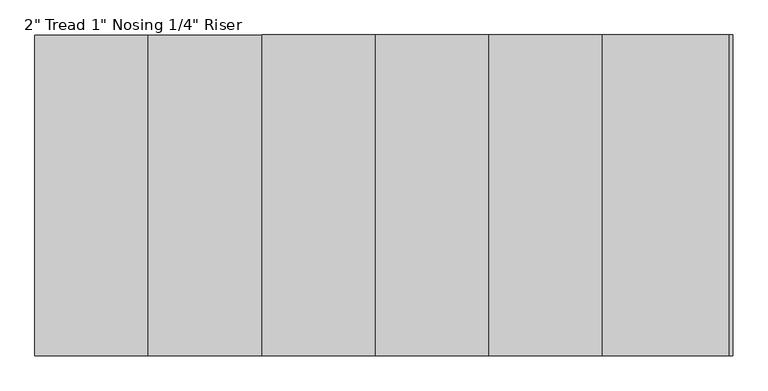
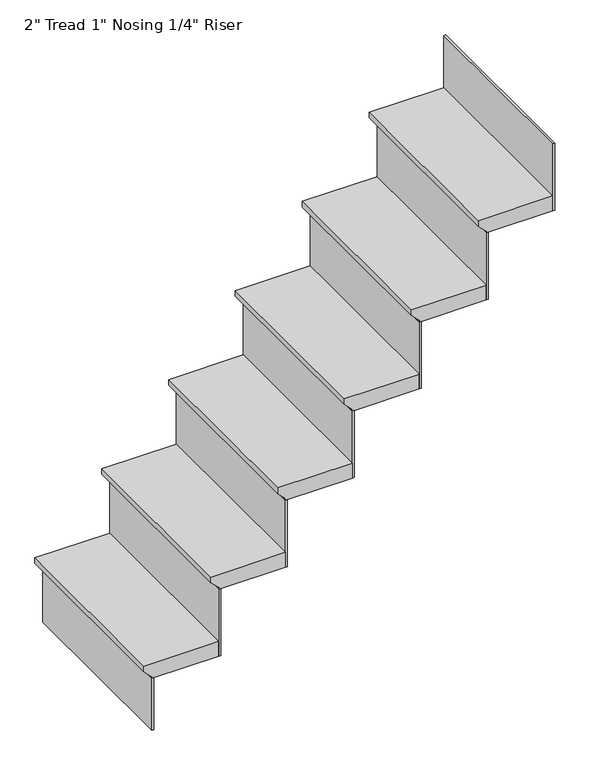
"""IFC4 building model written with IfcOpenShell, lengths in millimetres: stair flight geometry."""

from ifc_helpers import new_model, si_unit, origin, place, context, project, spatial, faceted_brep, source, transform, mapped, element, save


def stair_flight_4ab14130(model_context):
    return source(origin(), model_context, "Body", "Brep", [
        faceted_brep([(-5028.1409298, -3848.0779636, 209.55), (-5028.1409298, -3848.0779636, 228.6), (-5028.1409298, -3238.4779636, 228.6), (-5028.1409298, -3238.4779636, 209.55), (-5002.7409298, -3848.0779636, 184.15), (-5002.7409298, -3238.4779636, 184.15), (-4786.8409298, -3848.0779636, 228.6), (-4786.8409298, -3238.4779636, 228.6), (-5002.7409298, -3238.4779636, 177.8), (-4786.8409298, -3238.4779636, 177.8), (-4786.8409298, -3848.0779636, 177.8), (-5002.7409298, -3848.0779636, 177.8)], [[[0, 1, 2, 3]], [[4, 0, 3, 5]], [[2, 1, 6, 7]], [[8, 9, 10, 11]], [[2, 7, 9, 8, 5, 3]], [[8, 11, 4, 5]], [[6, 1, 0, 4, 11, 10]], [[7, 6, 10, 9]]]),
        faceted_brep([(-5002.7409298, -3848.0779636, 177.8), (-5002.7409298, -3848.0779636, 0.0), (-4996.3909298, -3848.0779636, 0.0), (-4996.3909298, -3848.0779636, 177.8), (-5002.7409298, -3238.4779636, 177.8), (-4996.3909298, -3238.4779636, 177.8), (-4996.3909298, -3238.4779636, 0.0), (-5002.7409298, -3238.4779636, 0.0)], [[[0, 1, 2, 3]], [[4, 5, 6, 7]], [[1, 0, 4, 7]], [[2, 1, 7, 6]], [[3, 2, 6, 5]], [[0, 3, 5, 4]]]),
        faceted_brep([(-4786.8409298, -3848.0779636, 406.4), (-4786.8409298, -3848.0779636, 177.8), (-4780.4909298, -3848.0779636, 177.8), (-4780.4909298, -3848.0779636, 406.4), (-4786.8409298, -3238.4779636, 406.4), (-4780.4909298, -3238.4779636, 406.4), (-4780.4909298, -3238.4779636, 177.8), (-4786.8409298, -3238.4779636, 177.8)], [[[0, 1, 2, 3]], [[4, 5, 6, 7]], [[1, 0, 4, 7]], [[2, 1, 7, 6]], [[3, 2, 6, 5]], [[0, 3, 5, 4]]]),
        faceted_brep([(-4812.2409298, -3238.4779636, 457.2), (-4812.2409298, -3848.0779636, 457.2), (-4570.9409298, -3848.0779636, 457.2), (-4570.9409298, -3238.4779636, 457.2), (-4786.8409298, -3238.4779636, 406.4), (-4570.9409298, -3238.4779636, 406.4), (-4570.9409298, -3848.0779636, 406.4), (-4786.8409298, -3848.0779636, 406.4), (-4786.8409298, -3238.4779636, 412.75), (-4812.2409298, -3238.4779636, 438.15), (-4786.8409298, -3848.0779636, 412.75), (-4812.2409298, -3848.0779636, 438.15)], [[[0, 1, 2, 3]], [[4, 5, 6, 7]], [[0, 3, 5, 4, 8, 9]], [[4, 7, 10, 8]], [[2, 1, 11, 10, 7, 6]], [[3, 2, 6, 5]], [[11, 1, 0, 9]], [[10, 11, 9, 8]]]),
        faceted_brep([(-4570.9409298, -3848.0779636, 635.0), (-4570.9409298, -3848.0779636, 406.4), (-4564.5909298, -3848.0779636, 406.4), (-4564.5909298, -3848.0779636, 635.0), (-4570.9409298, -3238.4779636, 635.0), (-4564.5909298, -3238.4779636, 635.0), (-4564.5909298, -3238.4779636, 406.4), (-4570.9409298, -3238.4779636, 406.4)], [[[0, 1, 2, 3]], [[4, 5, 6, 7]], [[1, 0, 4, 7]], [[2, 1, 7, 6]], [[3, 2, 6, 5]], [[0, 3, 5, 4]]]),
        faceted_brep([(-4596.3409298, -3238.4779636, 685.8), (-4596.3409298, -3848.0779636, 685.8), (-4355.0409298, -3848.0779636, 685.8), (-4355.0409298, -3238.4779636, 685.8), (-4570.9409298, -3238.4779636, 635.0), (-4355.0409298, -3238.4779636, 635.0), (-4355.0409298, -3848.0779636, 635.0), (-4570.9409298, -3848.0779636, 635.0), (-4570.9409298, -3238.4779636, 641.35), (-4596.3409298, -3238.4779636, 666.75), (-4570.9409298, -3848.0779636, 641.35), (-4596.3409298, -3848.0779636, 666.75)], [[[0, 1, 2, 3]], [[4, 5, 6, 7]], [[0, 3, 5, 4, 8, 9]], [[4, 7, 10, 8]], [[2, 1, 11, 10, 7, 6]], [[3, 2, 6, 5]], [[11, 1, 0, 9]], [[10, 11, 9, 8]]]),
        faceted_brep([(-4355.0409298, -3848.0779636, 863.6), (-4355.0409298, -3848.0779636, 635.0), (-4348.6909298, -3848.0779636, 635.0), (-4348.6909298, -3848.0779636, 863.6), (-4355.0409298, -3238.4779636, 863.6), (-4348.6909298, -3238.4779636, 863.6), (-4348.6909298, -3238.4779636, 635.0), (-4355.0409298, -3238.4779636, 635.0)], [[[0, 1, 2, 3]], [[4, 5, 6, 7]], [[1, 0, 4, 7]], [[2, 1, 7, 6]], [[3, 2, 6, 5]], [[0, 3, 5, 4]]]),
        faceted_brep([(-4380.4409298, -3238.4779636, 914.4), (-4380.4409298, -3848.0779636, 914.4), (-4139.1409298, -3848.0779636, 914.4), (-4139.1409298, -3238.4779636, 914.4), (-4355.0409298, -3238.4779636, 863.6), (-4139.1409298, -3238.4779636, 863.6), (-4139.1409298, -3848.0779636, 863.6), (-4355.0409298, -3848.0779636, 863.6), (-4355.0409298, -3238.4779636, 869.95), (-4380.4409298, -3238.4779636, 895.35), (-4355.0409298, -3848.0779636, 869.95), (-4380.4409298, -3848.0779636, 895.35)], [[[0, 1, 2, 3]], [[4, 5, 6, 7]], [[0, 3, 5, 4, 8, 9]], [[4, 7, 10, 8]], [[2, 1, 11, 10, 7, 6]], [[3, 2, 6, 5]], [[11, 1, 0, 9]], [[10, 11, 9, 8]]]),
        faceted_brep([(-4139.1409298, -3848.0779636, 1092.2), (-4139.1409298, -3848.0779636, 863.6), (-4132.7909298, -3848.0779636, 863.6), (-4132.7909298, -3848.0779636, 1092.2), (-4139.1409298, -3238.4779636, 1092.2), (-4132.7909298, -3238.4779636, 1092.2), (-4132.7909298, -3238.4779636, 863.6), (-4139.1409298, -3238.4779636, 863.6)], [[[0, 1, 2, 3]], [[4, 5, 6, 7]], [[1, 0, 4, 7]], [[2, 1, 7, 6]], [[3, 2, 6, 5]], [[0, 3, 5, 4]]]),
        faceted_brep([(-4164.5409298, -3238.4779636, 1143.0), (-4164.5409298, -3848.0779636, 1143.0), (-3923.2409298, -3848.0779636, 1143.0), (-3923.2409298, -3238.4779636, 1143.0), (-4139.1409298, -3238.4779636, 1092.2), (-3923.2409298, -3238.4779636, 1092.2), (-3923.2409298, -3848.0779636, 1092.2), (-4139.1409298, -3848.0779636, 1092.2), (-4139.1409298, -3238.4779636, 1098.55), (-4164.5409298, -3238.4779636, 1123.95), (-4139.1409298, -3848.0779636, 1098.55), (-4164.5409298, -3848.0779636, 1123.95)], [[[0, 1, 2, 3]], [[4, 5, 6, 7]], [[0, 3, 5, 4, 8, 9]], [[4, 7, 10, 8]], [[2, 1, 11, 10, 7, 6]], [[3, 2, 6, 5]], [[11, 1, 0, 9]], [[10, 11, 9, 8]]]),
        faceted_brep([(-3707.3409298, -3848.0779636, 1549.4), (-3707.3409298, -3848.0779636, 1320.8), (-3700.9909298, -3848.0779636, 1320.8), (-3700.9909298, -3848.0779636, 1549.4), (-3707.3409298, -3238.4779636, 1549.4), (-3700.9909298, -3238.4779636, 1549.4), (-3700.9909298, -3238.4779636, 1320.8), (-3707.3409298, -3238.4779636, 1320.8)], [[[0, 1, 2, 3]], [[4, 5, 6, 7]], [[1, 0, 4, 7]], [[2, 1, 7, 6]], [[3, 2, 6, 5]], [[0, 3, 5, 4]]]),
        faceted_brep([(-3923.2409298, -3848.0779636, 1320.8), (-3923.2409298, -3848.0779636, 1092.2), (-3916.8909298, -3848.0779636, 1092.2), (-3916.8909298, -3848.0779636, 1320.8), (-3923.2409298, -3238.4779636, 1320.8), (-3916.8909298, -3238.4779636, 1320.8), (-3916.8909298, -3238.4779636, 1092.2), (-3923.2409298, -3238.4779636, 1092.2)], [[[0, 1, 2, 3]], [[4, 5, 6, 7]], [[1, 0, 4, 7]], [[2, 1, 7, 6]], [[3, 2, 6, 5]], [[0, 3, 5, 4]]]),
        faceted_brep([(-3707.3409298, -3238.4779636, 1371.6), (-3732.7409298, -3238.4779636, 1371.6), (-3948.6409298, -3238.4779636, 1371.6), (-3948.6409298, -3848.0779636, 1371.6), (-3707.3409298, -3848.0779636, 1371.6), (-3732.7409298, -3238.4779636, 1320.8), (-3707.3409298, -3238.4779636, 1320.8), (-3707.3409298, -3848.0779636, 1320.8), (-3923.2409298, -3848.0779636, 1320.8), (-3923.2409298, -3238.4779636, 1320.8), (-3923.2409298, -3238.4779636, 1327.15), (-3948.6409298, -3238.4779636, 1352.55), (-3923.2409298, -3848.0779636, 1327.15), (-3948.6409298, -3848.0779636, 1352.55)], [[[0, 1, 2, 3, 4]], [[5, 6, 7, 8, 9]], [[1, 0, 6, 5]], [[2, 1, 5, 9, 10, 11]], [[9, 8, 12, 10]], [[4, 3, 13, 12, 8, 7]], [[0, 4, 7, 6]], [[13, 3, 2, 11]], [[12, 13, 11, 10]]]),
    ])


if __name__ == "__main__":
    model = new_model("IFC4")
    model_context = context("Model", 3, world=origin())
    ifc_project = project(units=[si_unit("LENGTHUNIT", "METRE", prefix="MILLI")], contexts=[model_context])
    site = spatial("IfcSite", under=ifc_project)
    building = spatial("IfcBuilding", under=site)
    placement = place(None, origin())
    stair_flight_shape = stair_flight_4ab14130(model_context)
    element("IfcStairFlight", 1, ObjectType="2\" Tread 1\" Nosing 1/4\" Riser", at=placement, inside=building, context=model_context, shape_type="MappedRepresentation", body=[
        mapped(stair_flight_shape, transform((0.0, 0.0, 0.0), x_axis=(1.0, 0.0, 0.0), y_axis=(0.0, 1.0, 0.0), z_axis=(0.0, 0.0, 1.0))),
    ])
    save(model, "model.ifc")
